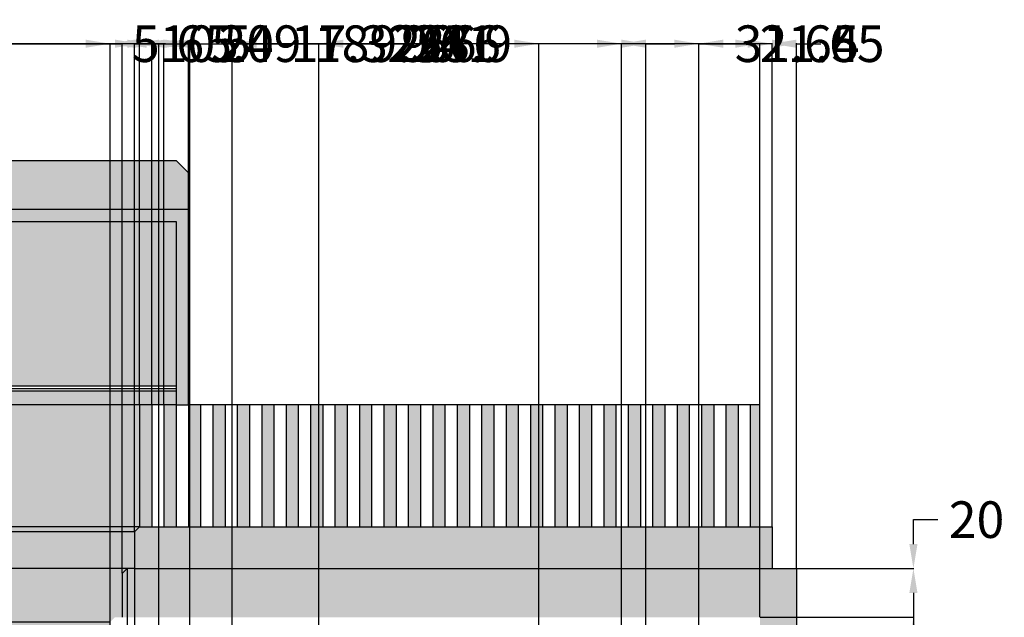
# Model space of a CAD drawing. Units: millimetres. Extents: x 131 to 845, y -20 to 1043.
# Tile 11 of 11: x 403 to 806, y 799 to 1043. Entities that reach past the tile are written whole.
import ezdxf

# ---------------------------------------------------------------- set-up
doc = ezdxf.new("R2010")
doc.units = ezdxf.units.MM
doc.header["$MEASUREMENT"] = 0
for name, color, linetype, lineweight in [('A-ANNO-DIMS', 2, 'Continuous', 18), ('A-ELEV', 7, 'Continuous', 25), ('A-ELEV-PATT', 7, 'Continuous', 13), ('A-WALL-PATT', 131, 'Continuous', 13)]:
    doc.layers.add(name, color=color, linetype=linetype, lineweight=lineweight)
doc.styles.get("Standard").update_dxf_attribs({"font": 'arial.ttf'})
doc.dimstyles.get("Standard").update_dxf_attribs({"dimtxt": 15, "dimasz": 10, "dimexe": 0.18, "dimexo": 0.0625, "dimgap": 5, "dimtad": 0, "dimtih": 1, "dimtoh": 1, "dimdec": 0, "dimzin": 0, "dimdsep": 46, "dimtxsty": 'Standard', "dimcen": 5, "dimadec": 0, "dimazin": 0, "dimtfac": 1, "dimtdec": 0, "dimtofl": 0, "dimtmove": 0, "dimatfit": 3, "dimfxl": 1, "dimtolj": 1, "dimtzin": 0, "dimarcsym": 0})

# ---------------------------------------------------------------- blocks, each defined once
blk = doc.blocks.new('*U1')
blk.add_line((0, 50), (0, 0))
blk = doc.blocks.new('*U2')
at = {"layer": 'A-ELEV', "color": 0, "linetype": 'ByBlock', "lineweight": -2, "transparency": 16777216}
for p in [(451.63, 835.67), (456.63, 835.67), (461.63, 835.67), (466.63, 835.67), (471.63, 835.67), (476.63, 835.67), (481.63, 835.67), (486.63, 835.67), (491.63, 835.67), (496.63, 835.67), (501.63, 835.67), (506.63, 835.67), (511.63, 835.67), (516.63, 835.67), (521.63, 835.67), (526.63, 835.67), (531.63, 835.67), (536.63, 835.67), (541.63, 835.67), (546.63, 835.67), (551.63, 835.67), (556.63, 835.67), (561.63, 835.67), (566.63, 835.67), (571.63, 835.67), (576.63, 835.67), (581.63, 835.67), (586.63, 835.67), (591.63, 835.67), (596.63, 835.67), (601.63, 835.67), (606.63, 835.67), (611.63, 835.67), (616.63, 835.67), (621.63, 835.67), (626.63, 835.67), (631.63, 835.67), (636.63, 835.67), (641.63, 835.67), (646.63, 835.67), (651.63, 835.67), (656.63, 835.67), (661.63, 835.67), (666.63, 835.67), (671.63, 835.67), (676.63, 835.67), (681.63, 835.67), (686.63, 835.67), (691.63, 835.67), (696.63, 835.67), (701.63, 835.67)]:
    blk.add_blockref('*U1', p, dxfattribs=at)
blk = doc.blocks.new('*D13')
at = {"layer": 'A-ANNO-DIMS', "color": 0, "lineweight": -2, "transparency": 16777216}
for p, q in [((210.58, 985.73), (210.58, 1033.7)), ((220.58, 1033.52), (444.01, 1033.52)), ((710.53, 1033.52), (487.1, 1033.52)), ((720.53, 818.66), (720.53, 1033.7))]:
    blk.add_line(p, q, dxfattribs=at)
at = {"layer": 'A-ANNO-DIMS', "color": 0, "transparency": 16777216}
for points in [[(220.58, 1035.18), (220.58, 1031.85), (210.58, 1033.52)], [(710.53, 1035.18), (710.53, 1031.85), (720.53, 1033.52)]]:
    blk.add_solid(points, dxfattribs=at)
at = {"layer": 'Defpoints', "color": 0, "transparency": 16777216}
for p in [(720.53, 1033.52), (210.58, 985.67), (720.53, 818.6)]:
    blk.add_point(p, dxfattribs=at)
at = {"layer": 'A-ANNO-DIMS', "color": 0, "transparency": 16777216, "insert": (465.56, 1033.52), "char_height": 15, "attachment_point": 5}
blk.add_mtext('\\A1;510', dxfattribs=at)
blk = doc.blocks.new('*D14')
at = {"layer": 'A-ANNO-DIMS', "color": 0, "lineweight": -2, "transparency": 16777216}
for p, q in [((210.52, 985.67), (162.55, 985.67)), ((162.73, 975.67), (162.73, 524.4)), ((162.73, 47.81), (162.73, 499.08)), ((459.5, 37.81), (162.55, 37.81))]:
    blk.add_line(p, q, dxfattribs=at)
at = {"layer": 'A-ANNO-DIMS', "color": 0, "transparency": 16777216}
for points in [[(161.06, 975.67), (164.4, 975.67), (162.73, 985.67)], [(161.06, 47.81), (164.4, 47.81), (162.73, 37.81)]]:
    blk.add_solid(points, dxfattribs=at)
at = {"layer": 'Defpoints', "color": 0, "transparency": 16777216}
for p in [(162.73, 985.67), (210.58, 985.67), (459.56, 37.81)]:
    blk.add_point(p, dxfattribs=at)
at = {"layer": 'A-ANNO-DIMS', "color": 0, "transparency": 16777216, "insert": (162.73, 511.74), "char_height": 15, "attachment_point": 5}
blk.add_mtext('\\A1;947.9', dxfattribs=at)
blk = doc.blocks.new('*D15')
at = {"layer": 'A-ANNO-DIMS', "color": 0, "lineweight": -2, "transparency": 16777216}
for p, q in [((210.58, 985.73), (210.58, 1033.7)), ((220.58, 1033.52), (304.79, 1033.52)), ((461.63, 1033.52), (377.43, 1033.52)), ((471.63, 965.73), (471.63, 1033.7))]:
    blk.add_line(p, q, dxfattribs=at)
at = {"layer": 'A-ANNO-DIMS', "color": 0, "transparency": 16777216}
for points in [[(220.58, 1035.18), (220.58, 1031.85), (210.58, 1033.52)], [(461.63, 1035.18), (461.63, 1031.85), (471.63, 1033.52)]]:
    blk.add_solid(points, dxfattribs=at)
at = {"layer": 'Defpoints', "color": 0, "transparency": 16777216}
for p in [(471.63, 1033.52), (210.58, 985.67), (471.63, 965.67)]:
    blk.add_point(p, dxfattribs=at)
at = {"layer": 'A-ANNO-DIMS', "color": 0, "transparency": 16777216, "insert": (341.11, 1033.52), "char_height": 15, "attachment_point": 5}
blk.add_mtext('\\A1;261.05', dxfattribs=at)
blk = doc.blocks.new('*D38')
at = {"layer": 'A-ANNO-DIMS', "color": 0, "lineweight": -2, "transparency": 16777216}
for p, q in [((439.56, 796.66), (439.56, 1033.7)), ((449.56, 1033.52), (550.85, 1033.52)), ((695.53, 1033.52), (594.24, 1033.52)), ((705.53, 798.66), (705.53, 1033.7))]:
    blk.add_line(p, q, dxfattribs=at)
at = {"layer": 'A-ANNO-DIMS', "color": 0, "transparency": 16777216}
for points in [[(449.56, 1035.18), (449.56, 1031.85), (439.56, 1033.52)], [(695.53, 1035.18), (695.53, 1031.85), (705.53, 1033.52)]]:
    blk.add_solid(points, dxfattribs=at)
at = {"layer": 'Defpoints', "color": 0, "transparency": 16777216}
for p in [(705.53, 1033.52), (705.53, 798.6), (439.56, 796.6)]:
    blk.add_point(p, dxfattribs=at)
at = {"layer": 'A-ANNO-DIMS', "color": 0, "transparency": 16777216, "insert": (572.55, 1033.52), "char_height": 15, "attachment_point": 5}
blk.add_mtext('\\A1;266', dxfattribs=at)
blk = doc.blocks.new('*D39')
at = {"layer": 'A-ANNO-DIMS', "color": 0, "lineweight": -2, "transparency": 16777216}
for p, q in [((444.56, 816.66), (444.56, 1033.7)), ((454.56, 1033.52), (560.85, 1033.52)), ((710.53, 1033.52), (604.24, 1033.52)), ((720.53, 818.66), (720.53, 1033.7))]:
    blk.add_line(p, q, dxfattribs=at)
at = {"layer": 'A-ANNO-DIMS', "color": 0, "transparency": 16777216}
for points in [[(454.56, 1035.18), (454.56, 1031.85), (444.56, 1033.52)], [(710.53, 1035.18), (710.53, 1031.85), (720.53, 1033.52)]]:
    blk.add_solid(points, dxfattribs=at)
at = {"layer": 'Defpoints', "color": 0, "transparency": 16777216}
for p in [(720.53, 1033.52), (720.53, 818.6), (444.56, 816.6)]:
    blk.add_point(p, dxfattribs=at)
at = {"layer": 'A-ANNO-DIMS', "color": 0, "transparency": 16777216, "insert": (582.55, 1033.52), "char_height": 15, "attachment_point": 5}
blk.add_mtext('\\A1;276', dxfattribs=at)
blk = doc.blocks.new('*D40')
at = {"layer": 'A-ANNO-DIMS', "color": 0, "lineweight": -2, "transparency": 16777216}
for p, q in [((720.6, 818.6), (768.56, 818.6)), ((768.38, 808.6), (768.38, 666.26)), ((768.38, 498.6), (768.38, 640.93)), ((720.6, 488.6), (768.56, 488.6))]:
    blk.add_line(p, q, dxfattribs=at)
at = {"layer": 'A-ANNO-DIMS', "color": 0, "transparency": 16777216}
for points in [[(766.72, 808.6), (770.05, 808.6), (768.38, 818.6)], [(766.72, 498.6), (770.05, 498.6), (768.38, 488.6)]]:
    blk.add_solid(points, dxfattribs=at)
at = {"layer": 'Defpoints', "color": 0, "transparency": 16777216}
for p in [(720.53, 818.6), (720.53, 488.6), (768.38, 488.6)]:
    blk.add_point(p, dxfattribs=at)
at = {"layer": 'A-ANNO-DIMS', "color": 0, "transparency": 16777216, "insert": (768.38, 653.6), "char_height": 15, "attachment_point": 5}
blk.add_mtext('\\A1;330', dxfattribs=at)
blk = doc.blocks.new('*D41')
at = {"layer": 'A-ANNO-DIMS', "color": 0, "lineweight": -2, "transparency": 16777216}
for p, q in [((768.38, 828.6), (768.38, 838.6)), ((768.38, 838.6), (778.38, 838.6)), ((720.6, 818.6), (768.56, 818.6)), ((705.6, 798.6), (768.56, 798.6)), ((768.38, 788.6), (768.38, 778.6))]:
    blk.add_line(p, q, dxfattribs=at)
at = {"layer": 'A-ANNO-DIMS', "color": 0, "transparency": 16777216}
for points in [[(766.72, 828.6), (770.05, 828.6), (768.38, 818.6)], [(766.72, 788.6), (770.05, 788.6), (768.38, 798.6)]]:
    blk.add_solid(points, dxfattribs=at)
at = {"layer": 'Defpoints', "color": 0, "transparency": 16777216}
for p in [(720.53, 818.6), (768.38, 818.6), (705.53, 798.6)]:
    blk.add_point(p, dxfattribs=at)
at = {"layer": 'A-ANNO-DIMS', "color": 0, "transparency": 16777216, "insert": (794.23, 838.6), "char_height": 15, "attachment_point": 5}
blk.add_mtext('\\A1;20', dxfattribs=at)
blk = doc.blocks.new('*D42')
at = {"layer": 'A-ANNO-DIMS', "color": 0, "lineweight": -2, "transparency": 16777216}
for p, q in [((459.56, 763.62), (459.56, 1033.7)), ((469.56, 1033.52), (518.83, 1033.52)), ((638.89, 1033.52), (589.63, 1033.52)), ((648.89, 763.62), (648.89, 1033.7))]:
    blk.add_line(p, q, dxfattribs=at)
at = {"layer": 'A-ANNO-DIMS', "color": 0, "transparency": 16777216}
for points in [[(469.56, 1035.18), (469.56, 1031.85), (459.56, 1033.52)], [(638.89, 1035.18), (638.89, 1031.85), (648.89, 1033.52)]]:
    blk.add_solid(points, dxfattribs=at)
at = {"layer": 'Defpoints', "color": 0, "transparency": 16777216}
for p in [(648.89, 1033.52), (459.56, 763.56), (648.89, 763.56)]:
    blk.add_point(p, dxfattribs=at)
at = {"layer": 'A-ANNO-DIMS', "color": 0, "transparency": 16777216, "insert": (554.23, 1033.52), "char_height": 15, "attachment_point": 5}
blk.add_mtext('\\A1;189.34', dxfattribs=at)
blk = doc.blocks.new('*D44')
at = {"layer": 'A-ANNO-DIMS', "color": 0, "lineweight": -2, "transparency": 16777216}
for p, q in [((429.56, 1033.52), (419.56, 1033.52)), ((439.56, 763.62), (439.56, 1033.7)), ((459.56, 763.62), (459.56, 1033.7)), ((469.56, 1033.52), (479.56, 1033.52))]:
    blk.add_line(p, q, dxfattribs=at)
at = {"layer": 'A-ANNO-DIMS', "color": 0, "transparency": 16777216}
for points in [[(429.56, 1035.18), (429.56, 1031.85), (439.56, 1033.52)], [(469.56, 1035.18), (469.56, 1031.85), (459.56, 1033.52)]]:
    blk.add_solid(points, dxfattribs=at)
at = {"layer": 'Defpoints', "color": 0, "transparency": 16777216}
for p in [(459.56, 1033.52), (439.56, 763.56), (459.56, 763.56)]:
    blk.add_point(p, dxfattribs=at)
at = {"layer": 'A-ANNO-DIMS', "color": 0, "transparency": 16777216, "insert": (495.4, 1033.52), "char_height": 15, "attachment_point": 5}
blk.add_mtext('\\A1;20', dxfattribs=at)
blk = doc.blocks.new('*D45')
at = {"layer": 'A-ANNO-DIMS', "color": 0, "lineweight": -2, "transparency": 16777216}
for p, q in [((162.73, 796.6), (162.73, 806.6)), ((162.73, 806.6), (172.73, 806.6)), ((439.5, 796.6), (162.55, 796.6)), ((162.73, 773.56), (162.73, 786.6)), ((459.5, 763.56), (162.55, 763.56))]:
    blk.add_line(p, q, dxfattribs=at)
at = {"layer": 'A-ANNO-DIMS', "color": 0, "transparency": 16777216}
for points in [[(161.06, 786.6), (164.4, 786.6), (162.73, 796.6)], [(161.06, 773.56), (164.4, 773.56), (162.73, 763.56)]]:
    blk.add_solid(points, dxfattribs=at)
at = {"layer": 'Defpoints', "color": 0, "transparency": 16777216}
for p in [(162.73, 796.6), (439.56, 796.6), (459.56, 763.56)]:
    blk.add_point(p, dxfattribs=at)
at = {"layer": 'A-ANNO-DIMS', "color": 0, "transparency": 16777216, "insert": (203, 806.6), "char_height": 15, "attachment_point": 5}
blk.add_mtext('\\A1;33.04', dxfattribs=at)
blk = doc.blocks.new('*D46')
at = {"layer": 'A-ANNO-DIMS', "color": 0, "lineweight": -2, "transparency": 16777216}
for p, q in [((648.89, 532.06), (648.89, 1033.7)), ((658.89, 1033.52), (670.53, 1033.52)), ((680.53, 513.66), (680.53, 1033.7)), ((680.53, 1033.52), (690.53, 1033.52))]:
    blk.add_line(p, q, dxfattribs=at)
at = {"layer": 'A-ANNO-DIMS', "color": 0, "transparency": 16777216}
for points in [[(658.89, 1035.18), (658.89, 1031.85), (648.89, 1033.52)], [(670.53, 1035.18), (670.53, 1031.85), (680.53, 1033.52)]]:
    blk.add_solid(points, dxfattribs=at)
at = {"layer": 'Defpoints', "color": 0, "transparency": 16777216}
for p in [(680.53, 1033.52), (648.89, 532), (680.53, 513.6)]:
    blk.add_point(p, dxfattribs=at)
at = {"layer": 'A-ANNO-DIMS', "color": 0, "transparency": 16777216, "insert": (720.81, 1033.52), "char_height": 15, "attachment_point": 5}
blk.add_mtext('\\A1;31.64', dxfattribs=at)
blk = doc.blocks.new('*D54')
at = {"layer": 'A-ANNO-DIMS', "color": 0, "lineweight": -2, "transparency": 16777216}
for p, q in [((525.05, 693.33), (525.05, 1033.7)), ((535.05, 1033.52), (554.33, 1033.52)), ((605.05, 1033.52), (585.76, 1033.52)), ((615.05, 693.33), (615.05, 1033.7))]:
    blk.add_line(p, q, dxfattribs=at)
at = {"layer": 'A-ANNO-DIMS', "color": 0, "transparency": 16777216}
for points in [[(535.05, 1035.18), (535.05, 1031.85), (525.05, 1033.52)], [(605.05, 1035.18), (605.05, 1031.85), (615.05, 1033.52)]]:
    blk.add_solid(points, dxfattribs=at)
at = {"layer": 'Defpoints', "color": 0, "transparency": 16777216}
for p in [(615.05, 1033.52), (525.05, 693.27), (615.05, 693.27)]:
    blk.add_point(p, dxfattribs=at)
at = {"layer": 'A-ANNO-DIMS', "color": 0, "transparency": 16777216, "insert": (570.05, 1033.52), "char_height": 15, "attachment_point": 5}
blk.add_mtext('\\A1;90', dxfattribs=at)
blk = doc.blocks.new('*D56')
at = {"layer": 'A-ANNO-DIMS', "color": 0, "lineweight": -2, "transparency": 16777216}
for p, q in [((449.56, 1033.52), (439.56, 1033.52)), ((459.56, 763.62), (459.56, 1033.7)), ((525.05, 693.33), (525.05, 1033.7)), ((535.05, 1033.52), (545.05, 1033.52))]:
    blk.add_line(p, q, dxfattribs=at)
at = {"layer": 'A-ANNO-DIMS', "color": 0, "transparency": 16777216}
for points in [[(449.56, 1035.18), (449.56, 1031.85), (459.56, 1033.52)], [(535.05, 1035.18), (535.05, 1031.85), (525.05, 1033.52)]]:
    blk.add_solid(points, dxfattribs=at)
at = {"layer": 'Defpoints', "color": 0, "transparency": 16777216}
for p in [(525.05, 1033.52), (459.56, 763.56), (525.05, 693.27)]:
    blk.add_point(p, dxfattribs=at)
at = {"layer": 'A-ANNO-DIMS', "color": 0, "transparency": 16777216, "insert": (492.3, 1033.52), "char_height": 15, "attachment_point": 5}
blk.add_mtext('\\A1;65.49', dxfattribs=at)
blk = doc.blocks.new('*D58')
at = {"layer": 'A-ANNO-DIMS', "color": 0, "lineweight": -2, "transparency": 16777216}
for p, q in [((525.05, 459.87), (525.05, 1033.7)), ((535.05, 1033.52), (554.33, 1033.52)), ((605.05, 1033.52), (585.76, 1033.52)), ((615.05, 459.87), (615.05, 1033.7))]:
    blk.add_line(p, q, dxfattribs=at)
at = {"layer": 'A-ANNO-DIMS', "color": 0, "transparency": 16777216}
for points in [[(535.05, 1035.18), (535.05, 1031.85), (525.05, 1033.52)], [(605.05, 1035.18), (605.05, 1031.85), (615.05, 1033.52)]]:
    blk.add_solid(points, dxfattribs=at)
at = {"layer": 'Defpoints', "color": 0, "transparency": 16777216}
for p in [(615.05, 1033.52), (525.05, 459.8), (615.05, 459.8)]:
    blk.add_point(p, dxfattribs=at)
at = {"layer": 'A-ANNO-DIMS', "color": 0, "transparency": 16777216, "insert": (570.05, 1033.52), "char_height": 15, "attachment_point": 5}
blk.add_mtext('\\A1;90', dxfattribs=at)
blk = doc.blocks.new('*D75')
at = {"layer": 'A-ANNO-DIMS', "color": 0, "lineweight": -2, "transparency": 16777216}
for p, q in [((462.24, 1033.52), (452.24, 1033.52)), ((472.24, 310.22), (472.24, 1033.7)), ((489.56, 300.22), (489.56, 1033.7)), ((499.56, 1033.52), (509.56, 1033.52))]:
    blk.add_line(p, q, dxfattribs=at)
at = {"layer": 'A-ANNO-DIMS', "color": 0, "transparency": 16777216}
for points in [[(462.24, 1035.18), (462.24, 1031.85), (472.24, 1033.52)], [(499.56, 1035.18), (499.56, 1031.85), (489.56, 1033.52)]]:
    blk.add_solid(points, dxfattribs=at)
at = {"layer": 'Defpoints', "color": 0, "transparency": 16777216}
for p in [(489.56, 1033.52), (472.24, 310.16), (489.56, 300.16)]:
    blk.add_point(p, dxfattribs=at)
at = {"layer": 'A-ANNO-DIMS', "color": 0, "transparency": 16777216, "insert": (539.08, 1033.52), "char_height": 15, "attachment_point": 5}
blk.add_mtext('\\A1;17.32', dxfattribs=at)
blk = doc.blocks.new('*D77')
at = {"layer": 'A-ANNO-DIMS', "color": 0, "lineweight": -2, "transparency": 16777216}
for p, q in [((648.88, 1033.52), (638.88, 1033.52)), ((658.88, 312.72), (658.88, 1033.7)), ((680.53, 300.22), (680.53, 1033.7)), ((690.53, 1033.52), (700.53, 1033.52))]:
    blk.add_line(p, q, dxfattribs=at)
at = {"layer": 'A-ANNO-DIMS', "color": 0, "transparency": 16777216}
for points in [[(648.88, 1035.18), (648.88, 1031.85), (658.88, 1033.52)], [(690.53, 1035.18), (690.53, 1031.85), (680.53, 1033.52)]]:
    blk.add_solid(points, dxfattribs=at)
at = {"layer": 'Defpoints', "color": 0, "transparency": 16777216}
for p in [(680.53, 1033.52), (658.88, 312.66), (680.53, 300.16)]:
    blk.add_point(p, dxfattribs=at)
at = {"layer": 'A-ANNO-DIMS', "color": 0, "transparency": 16777216, "insert": (731.03, 1033.52), "char_height": 15, "attachment_point": 5}
blk.add_mtext('\\A1;21.65', dxfattribs=at)
blk = doc.blocks.new('*D93')
at = {"layer": 'A-ANNO-DIMS', "color": 0, "lineweight": -2, "transparency": 16777216}
for p, q in [((162.73, 843.6), (162.73, 853.6)), ((162.73, 853.6), (172.73, 853.6)), ((449.5, 833.6), (162.55, 833.6)), ((449.5, 818.6), (162.55, 818.6)), ((162.73, 808.6), (162.73, 798.6))]:
    blk.add_line(p, q, dxfattribs=at)
at = {"layer": 'A-ANNO-DIMS', "color": 0, "transparency": 16777216}
for points in [[(161.06, 843.6), (164.4, 843.6), (162.73, 833.6)], [(161.06, 808.6), (164.4, 808.6), (162.73, 818.6)]]:
    blk.add_solid(points, dxfattribs=at)
at = {"layer": 'Defpoints', "color": 0, "transparency": 16777216}
for p in [(162.73, 833.6), (449.56, 833.6), (449.56, 818.6)]:
    blk.add_point(p, dxfattribs=at)
at = {"layer": 'A-ANNO-DIMS', "color": 0, "transparency": 16777216, "insert": (187.83, 853.6), "char_height": 15, "attachment_point": 5}
blk.add_mtext('\\A1;15', dxfattribs=at)
blk = doc.blocks.new('*D94')
at = {"layer": 'A-ANNO-DIMS', "color": 0, "lineweight": -2, "transparency": 16777216}
for p, q in [((162.73, 885.67), (162.73, 895.67)), ((162.73, 895.67), (172.73, 895.67)), ((451.57, 885.67), (162.55, 885.67)), ((162.73, 845.67), (162.73, 875.67)), ((451.57, 835.67), (162.55, 835.67))]:
    blk.add_line(p, q, dxfattribs=at)
at = {"layer": 'A-ANNO-DIMS', "color": 0, "transparency": 16777216}
for points in [[(161.06, 875.67), (164.4, 875.67), (162.73, 885.67)], [(161.06, 845.67), (164.4, 845.67), (162.73, 835.67)]]:
    blk.add_solid(points, dxfattribs=at)
at = {"layer": 'Defpoints', "color": 0, "transparency": 16777216}
for p in [(162.73, 885.67), (451.63, 885.67), (451.63, 835.67)]:
    blk.add_point(p, dxfattribs=at)
at = {"layer": 'A-ANNO-DIMS', "color": 0, "transparency": 16777216, "insert": (188.45, 895.67), "char_height": 15, "attachment_point": 5}
blk.add_mtext('\\A1;50', dxfattribs=at)
blk = doc.blocks.new('*D95')
at = {"layer": 'A-ANNO-DIMS', "color": 0, "lineweight": -2, "transparency": 16777216}
for p, q in [((441.63, 1033.52), (431.63, 1033.52)), ((451.63, 885.73), (451.63, 1033.7)), ((456.63, 885.73), (456.63, 1033.7)), ((466.63, 1033.52), (476.63, 1033.52))]:
    blk.add_line(p, q, dxfattribs=at)
at = {"layer": 'A-ANNO-DIMS', "color": 0, "transparency": 16777216}
for points in [[(441.63, 1035.18), (441.63, 1031.85), (451.63, 1033.52)], [(466.63, 1035.18), (466.63, 1031.85), (456.63, 1033.52)]]:
    blk.add_solid(points, dxfattribs=at)
at = {"layer": 'Defpoints', "color": 0, "transparency": 16777216}
for p in [(456.63, 1033.52), (451.63, 885.67), (456.63, 885.67)]:
    blk.add_point(p, dxfattribs=at)
at = {"layer": 'A-ANNO-DIMS', "color": 0, "transparency": 16777216, "insert": (486.6, 1033.52), "char_height": 15, "attachment_point": 5}
blk.add_mtext('\\A1;5', dxfattribs=at)
blk = doc.blocks.new('*D96')
at = {"layer": 'A-ANNO-DIMS', "color": 0, "lineweight": -2, "transparency": 16777216}
for p, q in [((446.63, 1033.52), (436.63, 1033.52)), ((456.63, 885.73), (456.63, 1033.7)), ((461.63, 885.73), (461.63, 1033.7)), ((471.63, 1033.52), (481.63, 1033.52))]:
    blk.add_line(p, q, dxfattribs=at)
at = {"layer": 'A-ANNO-DIMS', "color": 0, "transparency": 16777216}
for points in [[(446.63, 1035.18), (446.63, 1031.85), (456.63, 1033.52)], [(471.63, 1035.18), (471.63, 1031.85), (461.63, 1033.52)]]:
    blk.add_solid(points, dxfattribs=at)
at = {"layer": 'Defpoints', "color": 0, "transparency": 16777216}
for p in [(461.63, 1033.52), (456.63, 885.67), (461.63, 885.67)]:
    blk.add_point(p, dxfattribs=at)
at = {"layer": 'A-ANNO-DIMS', "color": 0, "transparency": 16777216, "insert": (491.6, 1033.52), "char_height": 15, "attachment_point": 5}
blk.add_mtext('\\A1;5', dxfattribs=at)
blk = doc.blocks.new('*D97')
at = {"layer": 'A-ANNO-DIMS', "color": 0, "lineweight": -2, "transparency": 16777216}
for p, q in [((451.63, 885.73), (451.63, 1033.7)), ((461.63, 1033.52), (548.13, 1033.52)), ((695.53, 1033.52), (609.03, 1033.52)), ((705.53, 885.73), (705.53, 1033.7))]:
    blk.add_line(p, q, dxfattribs=at)
at = {"layer": 'A-ANNO-DIMS', "color": 0, "transparency": 16777216}
for points in [[(461.63, 1035.18), (461.63, 1031.85), (451.63, 1033.52)], [(695.53, 1035.18), (695.53, 1031.85), (705.53, 1033.52)]]:
    blk.add_solid(points, dxfattribs=at)
at = {"layer": 'Defpoints', "color": 0, "transparency": 16777216}
for p in [(705.53, 1033.52), (451.63, 885.67), (705.53, 885.67)]:
    blk.add_point(p, dxfattribs=at)
at = {"layer": 'A-ANNO-DIMS', "color": 0, "transparency": 16777216, "insert": (578.58, 1033.52), "char_height": 15, "attachment_point": 5}
blk.add_mtext('\\A1;253.9', dxfattribs=at)
blk = doc.blocks.new('*D98')
at = {"layer": 'A-ANNO-DIMS', "color": 0, "lineweight": -2, "transparency": 16777216}
for p, q in [((449.56, 833.66), (449.56, 1033.7)), ((459.56, 1033.52), (559.8, 1033.52)), ((700.53, 1033.52), (600.3, 1033.52)), ((710.53, 835.73), (710.53, 1033.7))]:
    blk.add_line(p, q, dxfattribs=at)
at = {"layer": 'A-ANNO-DIMS', "color": 0, "transparency": 16777216}
for points in [[(459.56, 1035.18), (459.56, 1031.85), (449.56, 1033.52)], [(700.53, 1035.18), (700.53, 1031.85), (710.53, 1033.52)]]:
    blk.add_solid(points, dxfattribs=at)
at = {"layer": 'Defpoints', "color": 0, "transparency": 16777216}
for p in [(710.53, 1033.52), (710.53, 835.67), (449.56, 833.6)]:
    blk.add_point(p, dxfattribs=at)
at = {"layer": 'A-ANNO-DIMS', "color": 0, "transparency": 16777216, "insert": (580.05, 1033.52), "char_height": 15, "attachment_point": 5}
blk.add_mtext('\\A1;261', dxfattribs=at)
blk = doc.blocks.new('*D99')
at = {"layer": 'A-ANNO-DIMS', "color": 0, "lineweight": -2, "transparency": 16777216}
for p, q in [((449.56, 833.53), (449.56, -10.22)), ((446.56, 818.53), (446.56, -10.22)), ((436.56, -10.04), (426.56, -10.04)), ((459.56, -10.04), (469.56, -10.04))]:
    blk.add_line(p, q, dxfattribs=at)
at = {"layer": 'A-ANNO-DIMS', "color": 0, "transparency": 16777216}
for points in [[(436.56, -8.37), (436.56, -11.7), (446.56, -10.04)], [(459.56, -8.37), (459.56, -11.7), (449.56, -10.04)]]:
    blk.add_solid(points, dxfattribs=at)
at = {"layer": 'Defpoints', "color": 0, "transparency": 16777216}
for p in [(449.56, 833.6), (446.56, 818.6), (449.56, -10.04)]:
    blk.add_point(p, dxfattribs=at)
at = {"layer": 'A-ANNO-DIMS', "color": 0, "transparency": 16777216, "insert": (479.47, -10.04), "char_height": 15, "attachment_point": 5}
blk.add_mtext('\\A1;3', dxfattribs=at)
blk = doc.blocks.new('*D100')
at = {"layer": 'A-ANNO-DIMS', "color": 0, "lineweight": -2, "transparency": 16777216}
for p, q in [((695.53, 1033.52), (685.53, 1033.52)), ((705.53, 835.73), (705.53, 1033.7)), ((710.53, 835.73), (710.53, 1033.7)), ((720.53, 1033.52), (730.53, 1033.52))]:
    blk.add_line(p, q, dxfattribs=at)
at = {"layer": 'A-ANNO-DIMS', "color": 0, "transparency": 16777216}
for points in [[(695.53, 1035.18), (695.53, 1031.85), (705.53, 1033.52)], [(720.53, 1035.18), (720.53, 1031.85), (710.53, 1033.52)]]:
    blk.add_solid(points, dxfattribs=at)
at = {"layer": 'Defpoints', "color": 0, "transparency": 16777216}
for p in [(710.53, 1033.52), (705.53, 835.67), (710.53, 835.67)]:
    blk.add_point(p, dxfattribs=at)
at = {"layer": 'A-ANNO-DIMS', "color": 0, "transparency": 16777216, "insert": (740.51, 1033.52), "char_height": 15, "attachment_point": 5}
blk.add_mtext('\\A1;5', dxfattribs=at)

msp = doc.modelspace()

# ---------------------------------------------------------------- hatches: boundary and pattern name
at = {"layer": 'A-ELEV-PATT'}
h = msp.add_hatch(color=256, dxfattribs=at)
h.set_gradient(color1=(255, 255, 255), color2=(99, 100, 102), name='INVSPHERICAL')
h.paths.add_polyline_path([(471.6297, 965.6663), (471.6297, 980.6663), (466.6297, 985.6663), (210.5817, 985.6663), (210.5817, 965.6663)])
h = msp.add_hatch(color=256, dxfattribs=at)
h.set_gradient(color1=(255, 255, 255), color2=(99, 100, 102))
h.paths.add_polyline_path([(210.5817, 965.6663), (215.5817, 960.6663), (466.6297, 960.6663), (466.6297, 885.6663), (471.6297, 885.6663), (471.6297, 960.6663), (471.6297, 965.6663)])
at = {"layer": 'A-ELEV-PATT', "transparency": 33554681}
h = msp.add_hatch(color=256, dxfattribs=at)
h.set_gradient(color2=(60, 2, 17), name='INVSPHERICAL')
h.paths.add_polyline_path([(456.6296, 885.6663), (451.6297, 885.6663), (451.6297, 835.6663), (456.6296, 835.6663)])
h.paths.add_polyline_path([(466.6297, 885.6663), (461.6297, 885.6663), (461.6297, 835.6663), (466.6297, 835.6663)])
h.paths.add_polyline_path([(476.6297, 885.6663), (471.6297, 885.6663), (471.6297, 835.6663), (476.6297, 835.6663)])
h.paths.add_polyline_path([(481.6297, 835.6663), (486.6297, 835.6663), (486.6297, 885.6663), (481.6297, 885.6663)])
h.paths.add_polyline_path([(496.6297, 885.6663), (491.6297, 885.6663), (491.6297, 835.6663), (496.6297, 835.6663)])
h.paths.add_polyline_path([(506.6297, 885.6663), (501.6297, 885.6663), (501.6297, 835.6663), (506.6297, 835.6663)])
h.paths.add_polyline_path([(516.6297, 885.6663), (511.6297, 885.6663), (511.6297, 835.6663), (516.6297, 835.6663)])
h.paths.add_polyline_path([(521.6297, 835.6663), (526.6297, 835.6663), (526.6297, 885.6663), (521.6297, 885.6663)])
h.paths.add_polyline_path([(536.6297, 885.6663), (531.6297, 885.6663), (531.6297, 835.6663), (536.6297, 835.6663)])
h.paths.add_polyline_path([(541.6297, 835.6663), (546.6297, 835.6663), (546.6297, 885.6663), (541.6297, 885.6663)])
h.paths.add_polyline_path([(551.6297, 835.6663), (556.6297, 835.6663), (556.6297, 885.6663), (551.6297, 885.6663)])
h.paths.add_polyline_path([(566.6297, 885.6663), (561.6297, 885.6663), (561.6297, 835.6663), (566.6297, 835.6663)])
h.paths.add_polyline_path([(576.6297, 885.6663), (571.6297, 885.6663), (571.6297, 835.6663), (576.6297, 835.6663)])
h.paths.add_polyline_path([(581.6297, 835.6663), (586.6297, 835.6663), (586.6297, 885.6663), (581.6297, 885.6663)])
h.paths.add_polyline_path([(596.6297, 885.6663), (591.6297, 885.6663), (591.6297, 835.6663), (596.6297, 835.6663)])
h.paths.add_polyline_path([(601.6297, 835.6663), (606.6297, 835.6663), (606.6297, 885.6663), (601.6297, 885.6663)])
h.paths.add_polyline_path([(616.6297, 885.6663), (611.6297, 885.6663), (611.6297, 835.6663), (616.6297, 835.6663)])
h.paths.add_polyline_path([(621.6297, 835.6663), (626.6297, 835.6663), (626.6297, 885.6663), (621.6297, 885.6663)])
h.paths.add_polyline_path([(636.6297, 885.6663), (631.6297, 885.6663), (631.6297, 835.6663), (636.6297, 835.6663)])
h.paths.add_polyline_path([(641.6297, 835.6663), (646.6297, 835.6663), (646.6297, 885.6663), (641.6297, 885.6663)])
h.paths.add_polyline_path([(656.6297, 885.6663), (651.6297, 885.6663), (651.6297, 835.6663), (656.6297, 835.6663)])
h.paths.add_polyline_path([(661.6297, 835.6663), (666.6297, 835.6663), (666.6297, 885.6663), (661.6297, 885.6663)])
h.paths.add_polyline_path([(671.6297, 835.6663), (676.6297, 835.6663), (676.6297, 885.6663), (671.6297, 885.6663)])
h.paths.add_polyline_path([(686.6297, 885.6663), (681.6297, 885.6663), (681.6297, 835.6663), (686.6297, 835.6663)])
h.paths.add_polyline_path([(691.6297, 835.6663), (696.6297, 835.6663), (696.6297, 885.6663), (691.6297, 885.6663)])
h.paths.add_polyline_path([(705.5349, 885.6663), (701.6297, 885.6663), (701.6297, 835.6663), (705.5349, 835.6663)])
at = {"layer": 'A-ELEV-PATT'}
h = msp.add_hatch(color=256, dxfattribs=at)
h.set_gradient(color1=(255, 255, 255), color2=(147, 149, 152), name='CURVED')
h.paths.add_polyline_path([(451.6297, 835.6663), (449.5586, 833.5953), (449.5586, 818.5953), (710.5349, 818.5953), (710.5349, 835.6663), (705.5349, 835.6663)])
at = {"layer": 'A-WALL-PATT'}
h = msp.add_hatch(color=256, dxfattribs=at)
h.dxf.hatch_style = 1
h.paths.add_polyline_path([(449.5586, 833.5953), (451.6297, 835.6663), (451.6297, 885.6663), (466.6297, 885.6663), (466.6297, 891.3345), (330.6595, 891.3345), (330.6595, 856.8345), (292.1595, 856.8345), (292.1595, 798.4332), (336.1595, 798.4332), (336.1595, 178.4332), (246.1595, 178.4332), (246.1595, 798.4332), (290.1595, 798.4332), (290.1595, 856.8345), (259.6595, 856.8345), (255.6595, 860.8345), (255.6595, 927.8345), (290.1595, 927.8345), (290.1595, 960.6663), (216.2327, 960.6663), (216.2327, 60.3131), (459.5586, 60.3131), (459.5586, 97.8131), (459.5586, 252.07), (459.5586, 283.5561), (369.5586, 283.5561), (369.5586, 763.5561), (439.5586, 763.5561), (439.5586, 778.6714), (439.5586, 793.5953), (439.5586, 796.5953), (441.5586, 798.5953), (444.5586, 798.5953), (444.5586, 813.5953), (444.5586, 816.5953), (446.5586, 818.5953), (449.5586, 818.5953)])
h.paths.add_polyline_path([(466.6297, 960.6663), (292.1595, 960.6663), (292.1595, 927.8345), (326.6595, 927.8345), (330.6595, 923.8345), (330.6595, 893.3345), (466.6297, 893.3345)], flags=17)
h.paths.add_polyline_path([(720.5349, 813.5953), (720.5349, 818.5953), (710.5349, 818.5953), (449.5586, 818.5953), (446.5586, 818.5953), (444.5586, 816.5953), (444.5586, 813.5953), (444.5586, 798.5953), (705.5349, 798.5953), (705.5349, 513.5953), (705.5349, 498.5953), (680.5349, 498.5953), (680.5349, 488.5953), (705.5349, 488.5953), (720.5349, 488.5953), (720.5349, 513.5953)])
h.paths.add_polyline_path([(680.5349, 498.5953), (412.6606, 498.5953), (412.6606, 488.5953), (680.5349, 488.5953)])

# ---------------------------------------------------------------- linework, layer by layer
at = {"layer": 'A-ELEV'}
for p, q in [((210.5817, 985.6663), (466.6297, 985.6663)), ((466.6297, 985.6663), (471.6297, 980.6663)), ((471.6297, 980.6663), (471.6297, 965.6663)), ((471.6297, 965.6663), (210.5817, 965.6663)), ((471.6297, 960.6663), (471.6297, 965.6663)), ((215.5817, 960.6663), (466.6297, 960.6663)), ((466.6297, 960.6663), (466.6297, 885.6663)), ((471.6297, 885.6663), (471.6297, 960.6663)), ((330.6595, 893.3345), (466.6297, 893.3345)), ((330.6595, 892.3345), (466.6297, 892.3345)), ((330.6595, 891.3345), (466.6297, 891.3345)), ((466.6297, 885.6663), (451.6297, 885.6663)), ((466.6297, 885.6663), (471.6297, 885.6663)), ((705.5349, 885.6663), (471.6297, 885.6663)), ((705.5349, 835.6663), (705.5349, 885.6663)), ((451.6297, 835.6663), (449.5586, 833.5953)), ((451.6297, 835.6663), (705.5349, 835.6663)), ((705.5349, 835.6663), (710.5349, 835.6663)), ((710.5349, 835.6663), (710.5349, 818.5953)), ((449.5586, 833.5953), (449.5586, 818.5953)), ((446.5586, 818.5953), (444.5586, 816.5953)), ((449.5586, 818.5953), (446.5586, 818.5953)), ((449.5586, 818.5953), (710.5349, 818.5953)), ((449.5586, 818.5953), (449.5586, 818.5953)), ((710.5349, 818.5953), (720.5349, 818.5953)), ((720.5349, 818.5953), (720.5349, 813.5953)), ((444.5586, 816.5953), (444.5586, 813.5953)), ((444.5586, 813.5953), (444.5586, 798.5953)), ((720.5349, 813.5953), (720.5349, 513.5953))]:
    msp.add_line(p, q, dxfattribs=at)

# ---------------------------------------------------------------- block references
msp.add_blockref('*U2', (0, 0), dxfattribs=at)

# ---------------------------------------------------------------- dimensions: what is measured, and where the dimension line sits
at = {"layer": 'A-ANNO-DIMS'}
for base, p1, p2, override, picture, middle in [((720.5349, 1033.5163), (210.5817, 985.6663), (720.5349, 818.5953), {"dimdec": 0, "dimlfac": 1, "dimrnd": 0, "dimzin": 0, "dimdsep": 46, "dimlunit": 2}, '*D13', (465.5583, 1033.5163)), ((471.6297, 1033.5163), (210.5817, 985.6663), (471.6297, 965.6663), {"dimdec": 2, "dimlfac": 1, "dimrnd": 0, "dimzin": 0, "dimdsep": 46, "dimlunit": 2}, '*D15', (341.1057, 1033.5163)), ((459.5586, 1033.5163), (439.5586, 763.5561), (459.5586, 763.5561), {"dimdec": 0, "dimlfac": 1, "dimrnd": 0, "dimzin": 0, "dimdsep": 46, "dimlunit": 2}, '*D44', (495.4044, 1033.5163)), ((456.6296, 1033.5163), (451.6297, 885.6663), (456.6296, 885.6663), {"dimdec": 0, "dimlfac": 1, "dimrnd": 0, "dimzin": 0, "dimdsep": 46, "dimlunit": 2}, '*D95', (486.6024, 1033.5163)), ((461.6297, 1033.5163), (456.6296, 885.6663), (461.6297, 885.6663), {"dimdec": 0, "dimlfac": 1, "dimrnd": 0, "dimzin": 0, "dimdsep": 46, "dimlunit": 2}, '*D96', (491.6024, 1033.5163)), ((705.5349, 1033.5163), (439.5586, 796.5953), (705.5349, 798.5953), {"dimdec": 0, "dimlfac": 1, "dimrnd": 0, "dimzin": 0, "dimdsep": 46, "dimlunit": 2}, '*D38', (572.5467, 1033.5163)), ((525.0467, 1033.5163), (459.5586, 763.5561), (525.0467, 693.2667), {"dimdec": 2, "dimlfac": 1, "dimrnd": 0, "dimzin": 0, "dimdsep": 46, "dimlunit": 2}, '*D56', (492.3027, 1033.5163)), ((720.5349, 1033.5163), (444.5586, 816.5953), (720.5349, 818.5953), {"dimdec": 0, "dimlfac": 1, "dimrnd": 0, "dimzin": 0, "dimdsep": 46, "dimlunit": 2}, '*D39', (582.5467, 1033.5163)), ((710.5349, 1033.5163), (449.5586, 833.5953), (710.5349, 835.6663), {"dimdec": 0, "dimlfac": 1, "dimrnd": 0, "dimzin": 0, "dimdsep": 46, "dimlunit": 2}, '*D98', (580.0467, 1033.5163)), ((705.5349, 1033.5163), (451.6297, 885.6663), (705.5349, 885.6663), {"dimdec": 1, "dimlfac": 1, "dimrnd": 0, "dimzin": 0, "dimdsep": 46, "dimlunit": 2}, '*D97', (578.5823, 1033.5163)), ((489.5586, 1033.5163), (472.2381, 310.1596), (489.5586, 300.1596), {"dimdec": 2, "dimlfac": 1, "dimrnd": 0, "dimzin": 0, "dimdsep": 46, "dimlunit": 2}, '*D75', (539.0845, 1033.5163)), ((648.8943, 1033.5163), (459.5586, 763.5561), (648.8943, 763.5561), {"dimdec": 2, "dimlfac": 1, "dimrnd": 0, "dimzin": 0, "dimdsep": 46, "dimlunit": 2}, '*D42', (554.2265, 1033.5163)), ((615.0467, 1033.5163), (525.0467, 693.2667), (615.0467, 693.2667), {"dimdec": 0, "dimlfac": 1, "dimrnd": 0, "dimzin": 0, "dimdsep": 46, "dimlunit": 2}, '*D54', (570.0467, 1033.5163)), ((615.0467, 1033.5163), (525.0467, 459.8046), (615.0467, 459.8046), {"dimdec": 0, "dimlfac": 1, "dimrnd": 0, "dimzin": 0, "dimdsep": 46, "dimlunit": 2}, '*D58', (570.0467, 1033.5163)), ((680.5349, 1033.5163), (658.8842, 312.6596), (680.5349, 300.1596), {"dimdec": 2, "dimlfac": 1, "dimrnd": 0, "dimzin": 0, "dimdsep": 46, "dimlunit": 2}, '*D77', (731.0277, 1033.5163)), ((680.5349, 1033.5163), (648.8943, 532.0012), (680.5349, 513.5953), {"dimdec": 2, "dimlfac": 1, "dimrnd": 0, "dimzin": 0, "dimdsep": 46, "dimlunit": 2}, '*D46', (720.8077, 1033.5163)), ((710.5349, 1033.5163), (705.5349, 835.6663), (710.5349, 835.6663), {"dimdec": 0, "dimlfac": 1, "dimrnd": 0, "dimzin": 0, "dimdsep": 46, "dimlunit": 2}, '*D100', (740.5076, 1033.5163)), ((449.5586, -10.0369), (446.5586, 818.5953), (449.5586, 833.5953), {"dimdec": 0, "dimlfac": 1, "dimrnd": 0, "dimzin": 0, "dimdsep": 46, "dimlunit": 2}, '*D99', (479.4699, -10.0369))]:
    dim = msp.add_linear_dim(base=base, p1=p1, p2=p2, dimstyle='Standard', override=override, dxfattribs=at)
    dim.commit()
    dim.dimension.update_dxf_attribs({"geometry": picture, "text_midpoint": middle})
for base, p1, p2, override, picture, middle in [((162.7317, 985.6663), (459.5586, 37.8131), (210.5817, 985.6663), {"dimdec": 1, "dimlfac": 1, "dimrnd": 0, "dimzin": 0, "dimdsep": 46, "dimlunit": 2}, '*D14', (162.7317, 511.7397)), ((162.7317, 885.6663), (451.6297, 835.6663), (451.6297, 885.6663), {"dimdec": 0, "dimlfac": 1, "dimrnd": 0, "dimzin": 0, "dimdsep": 46, "dimlunit": 2}, '*D94', (188.4496, 895.6663)), ((162.7317, 833.5953), (449.5586, 818.5953), (449.5586, 833.5953), {"dimdec": 0, "dimlfac": 1, "dimrnd": 0, "dimzin": 0, "dimdsep": 46, "dimlunit": 2}, '*D93', (187.8254, 853.5953)), ((768.3849, 818.5953), (705.5349, 798.5953), (720.5349, 818.5953), {"dimdec": 0, "dimlfac": 1, "dimrnd": 0, "dimzin": 0, "dimdsep": 46, "dimlunit": 2}, '*D41', (794.2307, 838.5953)), ((768.3849, 488.5953), (720.5349, 818.5953), (720.5349, 488.5953), {"dimdec": 0, "dimlfac": 1, "dimrnd": 0, "dimzin": 0, "dimdsep": 46, "dimlunit": 2}, '*D40', (768.3849, 653.5953)), ((162.7317, 796.5953), (459.5586, 763.5561), (439.5586, 796.5953), {"dimdec": 2, "dimlfac": 1, "dimrnd": 0, "dimzin": 0, "dimdsep": 46, "dimlunit": 2}, '*D45', (203.0045, 806.5953))]:
    dim = msp.add_linear_dim(base=base, p1=p1, p2=p2, angle=90, dimstyle='Standard', override=override, dxfattribs=at)
    dim.commit()
    dim.dimension.update_dxf_attribs({"geometry": picture, "text_midpoint": middle})

doc.saveas('drawing.dxf')
